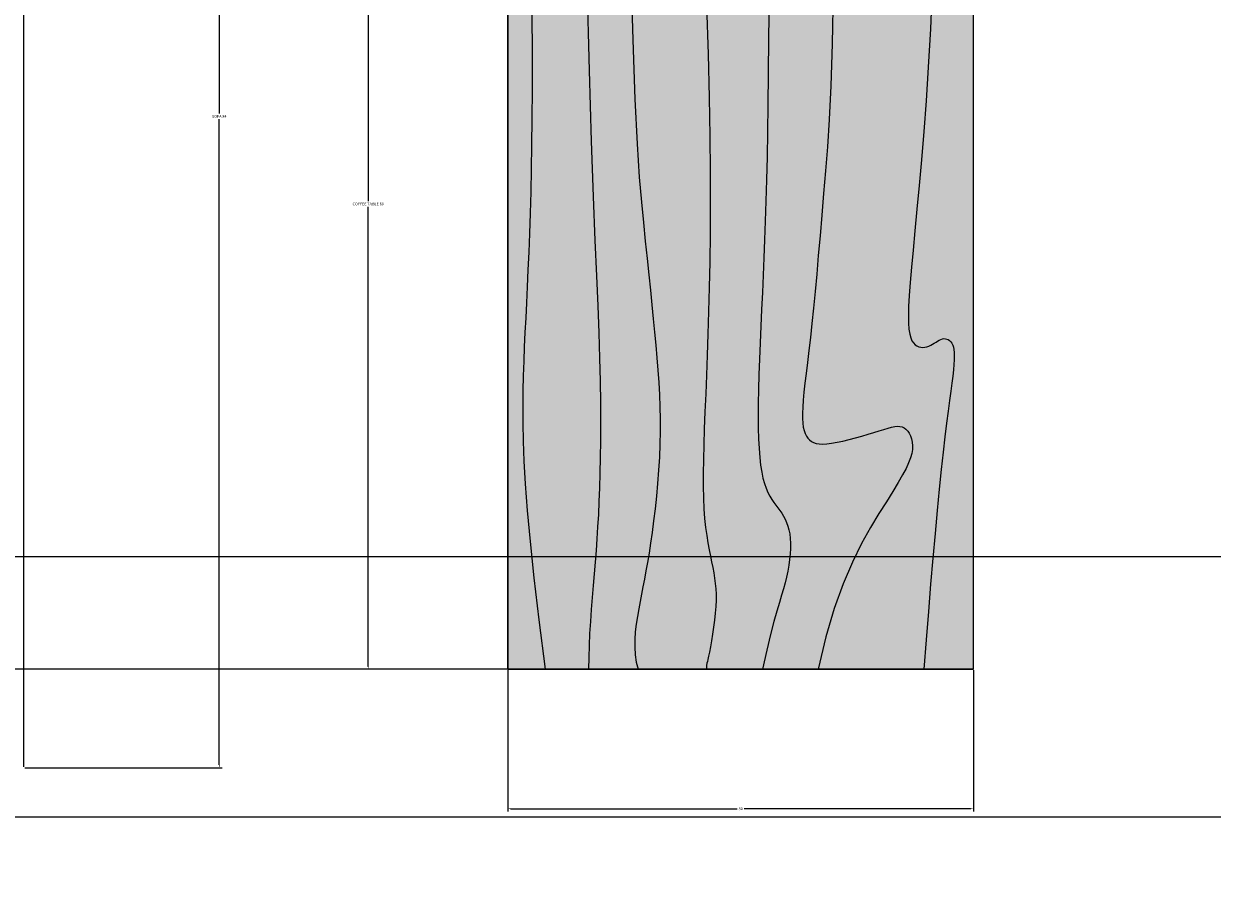
# Model space of a CAD drawing. Units: inches. Extents: x 1201 to 1754, y 247 to 775.
# Tile 3 of 10: x 1305 to 1382, y 435 to 491. Entities that reach past the tile are written whole.
import ezdxf

# ---------------------------------------------------------------- set-up
doc = ezdxf.new("R2010")
doc.units = ezdxf.units.IN
for name, color, linetype, lineweight in [('A-ANNO-DIMS', 2, 'Continuous', 18), ('A-FURN', 8, 'Continuous', 18), ('A-FURN-PATT', 9, 'Continuous', 13)]:
    doc.layers.add(name, color=color, linetype=linetype, lineweight=lineweight)
doc.styles.get("Standard").update_dxf_attribs({"font": 'arial.ttf'})
doc.dimstyles.get("Standard").update_dxf_attribs({"dimtxt": 0.18, "dimasz": 0.18, "dimexe": 0.18, "dimexo": 0.0625, "dimgap": 0.09, "dimtad": 0, "dimtih": 1, "dimtoh": 1, "dimdec": 4, "dimzin": 0, "dimdsep": 46, "dimtxsty": 'Standard', "dimcen": 0.09, "dimadec": 0, "dimazin": 0, "dimtfac": 1, "dimtdec": 4, "dimtofl": 0, "dimtmove": 0, "dimatfit": 3, "dimfxl": 1, "dimtolj": 1, "dimtzin": 0, "dimarcsym": 0})

# ---------------------------------------------------------------- blocks, each defined once
blk = doc.blocks.new('Table - Rectangular Woodgrain 60 x 30 in.')
for p, q in [((0, 0), (0, -30)), ((60, 0), (0, 0)), ((60, -30), (60, 0)), ((0, -30), (60, -30))]:
    blk.add_line(p, q)
for points in [[(0, -2.4), (4.8155, -2.418), (9.0302, -2.4688), (12.709, -2.5477), (15.9167, -2.65), (18.7181, -2.7711), (21.1781, -2.9063), (23.3616, -3.0508), (25.3333, -3.2), (27.1477, -3.3495), (28.8172, -3.4958), (30.3437, -3.636), (31.7291, -3.7667), (32.9756, -3.8849), (34.0849, -3.9875), (35.059, -4.0714), (35.9, -4.1334), (36.6114, -4.1711), (37.2041, -4.1854), (37.6906, -4.1779), (38.0833, -4.15), (38.3948, -4.1034), (38.6375, -4.0396), (38.8239, -3.9602), (38.9666, -3.8667), (39.0764, -3.7608), (39.1573, -3.6448), (39.2116, -3.521), (39.2416, -3.3917), (39.2498, -3.2593), (39.2385, -3.1261), (39.21, -2.9944), (39.1666, -2.8667), (39.111, -2.7447), (39.0468, -2.6281), (38.978, -2.5163), (38.9083, -2.4083), (38.8418, -2.3035), (38.7823, -2.201), (38.7337, -2.1001), (38.7, -2), (38.6844, -1.9003), (38.6875, -1.8021), (38.7094, -1.707), (38.75, -1.6167), (38.8094, -1.5326), (38.8875, -1.4563), (38.9844, -1.3893), (39.1, -1.3333), (39.2351, -1.2896), (39.3937, -1.2583), (39.5804, -1.2396), (39.8, -1.2333), (40.057, -1.2396), (40.3562, -1.2583), (40.7023, -1.2896), (41.1, -1.3333), (41.5547, -1.3895), (42.0755, -1.4573), (42.6721, -1.5361), (43.3542, -1.625), (44.1316, -1.7233), (45.014, -1.8302), (46.0114, -1.9449), (47.1333, -2.0667), (48.3862, -2.1947), (49.7625, -2.3281), (51.2513, -2.4663), (52.8416, -2.6083), (54.5226, -2.7535), (56.2833, -2.9011), (58.1127, -3.0501), (60, -3.2)], [(0, -9.2), (6.5759, -9.0858), (11.9385, -9.0365), (16.2527, -9.0418), (19.6833, -9.0917), (22.3952, -9.1759), (24.5531, -9.2844), (26.322, -9.4069), (27.8666, -9.5333), (29.3241, -9.6553), (30.7203, -9.7719), (32.0532, -9.8837), (33.3208, -9.9917), (34.5213, -10.0965), (35.6526, -10.199), (36.7128, -10.2999), (37.7, -10.4), (38.6129, -10.4996), (39.4531, -10.5969), (40.223, -10.6895), (40.925, -10.775), (41.5613, -10.8512), (42.1344, -10.9156), (42.6465, -10.966), (43.1, -11), (43.4976, -11.0158), (43.8437, -11.0136), (44.143, -10.9942), (44.4, -10.9583), (44.6195, -10.9069), (44.8062, -10.8406), (44.9648, -10.7603), (45.1, -10.6667), (45.2155, -10.5598), (45.3114, -10.4365), (45.3871, -10.2929), (45.4416, -10.125), (45.4743, -9.929), (45.4844, -9.7011), (45.4709, -9.4371), (45.4333, -9.1333), (45.3716, -8.7883), (45.2896, -8.4104), (45.1919, -8.0107), (45.0833, -7.6), (44.9685, -7.1893), (44.8521, -6.7896), (44.7388, -6.4117), (44.6333, -6.0667), (44.54, -5.7628), (44.4614, -5.4979), (44.4001, -5.2675), (44.3583, -5.0667), (44.3384, -4.8909), (44.3427, -4.7354), (44.3736, -4.5956), (44.4333, -4.4667), (44.5236, -4.3453), (44.6427, -4.2333), (44.7884, -4.1339), (44.9583, -4.05), (45.1501, -3.9849), (45.3614, -3.9417), (45.59, -3.9234), (45.8333, -3.9333), (46.0915, -3.9749), (46.3734, -4.0531), (46.6906, -4.1736), (47.0542, -4.3417), (47.4756, -4.5629), (47.9661, -4.8427), (48.5372, -5.1866), (49.2, -5.6), (49.9676, -6.0844), (50.8594, -6.625), (51.8965, -7.2031), (53.1, -7.8), (54.491, -8.3969), (56.0906, -8.975), (57.9199, -9.5156), (60, -10)], [(0, -12.8), (5.1847, -12.9322), (9.6213, -13.0323), (13.3963, -13.1059), (16.5958, -13.1583), (19.3063, -13.1952), (21.614, -13.2219), (23.6054, -13.2439), (25.3666, -13.2667), (26.9728, -13.2947), (28.4531, -13.3281), (29.8256, -13.3663), (31.1083, -13.4083), (32.3191, -13.4535), (33.476, -13.501), (34.597, -13.5501), (35.7, -13.6), (36.7984, -13.6497), (37.8875, -13.6979), (38.9578, -13.743), (40, -13.7833), (41.0047, -13.8174), (41.9625, -13.8438), (42.864, -13.8607), (43.7, -13.8667), (44.4631, -13.8604), (45.1552, -13.8417), (45.7801, -13.8104), (46.3416, -13.7667), (46.8439, -13.7104), (47.2906, -13.6417), (47.6858, -13.5604), (48.0333, -13.4667), (48.3375, -13.3608), (48.6042, -13.2448), (48.8396, -13.121), (49.05, -12.9917), (49.2417, -12.8593), (49.4208, -12.7261), (49.5937, -12.5944), (49.7667, -12.4667), (49.9452, -12.3451), (50.1323, -12.2313), (50.3303, -12.1268), (50.5416, -12.0333), (50.7686, -11.9524), (51.0135, -11.8854), (51.2788, -11.8341), (51.5666, -11.8), (51.8785, -11.7843), (52.2116, -11.7865), (52.562, -11.8059), (52.926, -11.8417), (53.2998, -11.8931), (53.6795, -11.9594), (54.0614, -12.0397), (54.4416, -12.1333), (54.8223, -12.2401), (55.2293, -12.3625), (55.6942, -12.5037), (56.2489, -12.6667), (56.9251, -12.8547), (57.7545, -13.0708), (58.7689, -13.3182), (60, -13.6)], [(0, -18), (5.124, -17.7273), (9.6609, -17.5057), (13.6705, -17.3303), (17.2125, -17.1958), (20.3467, -17.0973), (23.1328, -17.0297), (25.6307, -16.9878), (27.9, -16.9667), (29.9928, -16.9617), (31.9302, -16.9703), (33.7254, -16.9907), (35.3917, -17.0208), (36.9423, -17.0588), (38.3906, -17.1026), (39.7499, -17.1503), (41.0333, -17.2), (42.2519, -17.2496), (43.4073, -17.2969), (44.4986, -17.3395), (45.525, -17.375), (46.4858, -17.4012), (47.3802, -17.4156), (48.2074, -17.416), (48.9667, -17.4), (49.6583, -17.3662), (50.2872, -17.3167), (50.8595, -17.2547), (51.3812, -17.1833), (51.8584, -17.1057), (52.2971, -17.025), (52.7034, -16.9443), (53.0833, -16.8667), (53.443, -16.7951), (53.789, -16.7313), (54.128, -16.6768), (54.4666, -16.6334), (54.8115, -16.6024), (55.1693, -16.5854), (55.5465, -16.5841), (55.95, -16.6), (56.3828, -16.6337), (56.8346, -16.6823), (57.2915, -16.7418), (57.7396, -16.8084), (58.165, -16.878), (58.5539, -16.9469), (58.8924, -17.0111), (59.1666, -17.0667), (59.3679, -17.1107), (59.5078, -17.1438), (59.6032, -17.1675), (59.6708, -17.1833), (59.7275, -17.193), (59.7901, -17.1979), (59.8753, -17.1998), (60, -17.2)], [(0, -22.4), (8.0098, -22.2501), (14.4094, -22.1011), (19.4168, -21.9535), (23.25, -21.8083), (26.1269, -21.6663), (28.2656, -21.5281), (29.884, -21.3947), (31.2, -21.2667), (32.3967, -21.1448), (33.5172, -21.0292), (34.5697, -20.9198), (35.5625, -20.8167), (36.5037, -20.7198), (37.4015, -20.6292), (38.2642, -20.5448), (39.1, -20.4667), (39.9164, -20.3951), (40.7187, -20.3313), (41.5117, -20.2768), (42.3, -20.2333), (43.0883, -20.2024), (43.8812, -20.1854), (44.6836, -20.1841), (45.5, -20.2), (46.3328, -20.234), (47.1747, -20.2844), (48.0163, -20.3488), (48.8479, -20.425), (49.66, -20.5106), (50.4429, -20.6031), (51.1872, -20.7004), (51.8833, -20.8), (52.5246, -20.8999), (53.1166, -20.9995), (53.6681, -21.0983), (54.1875, -21.1958), (54.6834, -21.2919), (55.1646, -21.3859), (55.6394, -21.4777), (56.1167, -21.5667), (56.6028, -21.6515), (57.0961, -21.7266), (57.5929, -21.7852), (58.0896, -21.8208), (58.5823, -21.8268), (59.0674, -21.7964), (59.5412, -21.723), (60, -21.6)], [(0, -25.2), (8.6355, -25.0504), (15.7026, -24.9031), (21.4049, -24.7606), (25.9458, -24.625), (29.529, -24.4988), (32.3578, -24.3844), (34.6359, -24.284), (36.5667, -24.2), (38.3213, -24.1341), (39.9417, -24.0854), (41.437, -24.0523), (42.8167, -24.0333), (44.0901, -24.0268), (45.2667, -24.0313), (46.3557, -24.0451), (47.3667, -24.0667), (48.309, -24.0947), (49.1928, -24.1287), (50.0284, -24.168), (50.826, -24.2125), (51.5959, -24.2617), (52.3483, -24.3151), (53.0935, -24.3725), (53.8417, -24.4334), (54.6009, -24.497), (55.3699, -24.561), (56.1454, -24.6226), (56.9239, -24.6792), (57.7021, -24.7279), (58.4764, -24.7662), (59.2435, -24.7911), (60, -24.8)], [(0, -28.8), (5.6867, -28.6681), (10.45, -28.5698), (14.407, -28.5012), (17.675, -28.4584), (20.3711, -28.4374), (22.6125, -28.4344), (24.5164, -28.4455), (26.2, -28.4667), (27.762, -28.4947), (29.2276, -28.5281), (30.6033, -28.5663), (31.8958, -28.6084), (33.1118, -28.6535), (34.2578, -28.7011), (35.3405, -28.7501), (36.3666, -28.8), (37.3443, -28.8497), (38.288, -28.8974), (39.2137, -28.9412), (40.1375, -28.9792), (41.0753, -29.0093), (42.0432, -29.0297), (43.0572, -29.0384), (44.1333, -29.0333), (45.2936, -29.0114), (46.5843, -28.9641), (48.0579, -28.8816), (49.7666, -28.7542), (51.7629, -28.5721), (54.0989, -28.3255), (56.8272, -28.0048), (60, -27.6)]]:
    blk.add_lwpolyline(points)
blk = doc.blocks.new('*D35')
at = {"layer": 'A-ANNO-DIMS', "color": 0, "lineweight": -2, "transparency": 16777216}
for p, q in [((1336.149, 509.584), (1327.031, 509.584)), ((1327.211, 509.404), (1327.211, 479.767)), ((1327.211, 449.764), (1327.211, 479.401)), ((1336.149, 449.584), (1327.031, 449.584))]:
    blk.add_line(p, q, dxfattribs=at)
at = {"layer": 'A-ANNO-DIMS', "color": 0, "transparency": 16777216}
for points in [[(1327.181, 509.404), (1327.241, 509.404), (1327.211, 509.584)], [(1327.181, 449.764), (1327.241, 449.764), (1327.211, 449.584)]]:
    blk.add_solid(points, dxfattribs=at)
at = {"layer": 'Defpoints', "color": 0, "transparency": 16777216}
for p in [(1336.211, 509.584), (1327.211, 449.584), (1336.211, 449.584)]:
    blk.add_point(p, dxfattribs=at)
at = {"layer": 'A-ANNO-DIMS', "color": 0, "transparency": 16777216, "insert": (1327.211, 479.584), "char_height": 0.18, "attachment_point": 5}
blk.add_mtext('\\A1;COFFEE TABLE 60', dxfattribs=at)
blk = doc.blocks.new('*D36')
at = {"layer": 'A-ANNO-DIMS', "color": 0, "lineweight": -2, "transparency": 16777216}
for p, q in [((1336.211, 449.521), (1336.211, 440.404)), ((1366.211, 449.521), (1366.211, 440.404)), ((1336.391, 440.584), (1350.993, 440.584)), ((1366.031, 440.584), (1351.43, 440.584))]:
    blk.add_line(p, q, dxfattribs=at)
at = {"layer": 'A-ANNO-DIMS', "color": 0, "transparency": 16777216}
for points in [[(1336.391, 440.614), (1336.391, 440.554), (1336.211, 440.584)], [(1366.031, 440.614), (1366.031, 440.554), (1366.211, 440.584)]]:
    blk.add_solid(points, dxfattribs=at)
at = {"layer": 'Defpoints', "color": 0, "transparency": 16777216}
for p in [(1336.211, 449.584), (1366.211, 449.584), (1366.211, 440.584)]:
    blk.add_point(p, dxfattribs=at)
at = {"layer": 'A-ANNO-DIMS', "color": 0, "transparency": 16777216, "insert": (1351.211, 440.584), "char_height": 0.18, "attachment_point": 5}
blk.add_mtext('\\A1;30', dxfattribs=at)
blk = doc.blocks.new('*D37')
at = {"layer": 'A-ANNO-DIMS', "color": 0, "lineweight": -2, "transparency": 16777216}
for p, q in [((1305.079, 527.227), (1317.797, 527.227)), ((1317.617, 527.047), (1317.617, 485.41)), ((1317.617, 443.407), (1317.617, 485.044)), ((1305.079, 443.227), (1317.797, 443.227))]:
    blk.add_line(p, q, dxfattribs=at)
at = {"layer": 'A-ANNO-DIMS', "color": 0, "transparency": 16777216}
for points in [[(1317.587, 527.047), (1317.647, 527.047), (1317.617, 527.227)], [(1317.587, 443.407), (1317.647, 443.407), (1317.617, 443.227)]]:
    blk.add_solid(points, dxfattribs=at)
at = {"layer": 'Defpoints', "color": 0, "transparency": 16777216}
for p in [(1305.017, 527.227), (1317.617, 527.227), (1305.017, 443.227)]:
    blk.add_point(p, dxfattribs=at)
at = {"layer": 'A-ANNO-DIMS', "color": 0, "transparency": 16777216, "insert": (1317.617, 485.227), "char_height": 0.18, "attachment_point": 5}
blk.add_mtext('\\A1;SOFA 84', dxfattribs=at)
blk = doc.blocks.new('*D59')
at = {"layer": 'A-ANNO-DIMS', "color": 0, "lineweight": -2, "transparency": 16777216}
for p, q in [((1255.521, 418.004), (1255.521, 775.136)), ((1405.521, 418.004), (1405.521, 775.136)), ((1255.701, 774.956), (1330.241, 774.956)), ((1405.341, 774.956), (1330.801, 774.956))]:
    blk.add_line(p, q, dxfattribs=at)
at = {"layer": 'A-ANNO-DIMS', "color": 0, "transparency": 16777216}
for points in [[(1255.701, 774.986), (1255.701, 774.926), (1255.521, 774.956)], [(1405.341, 774.986), (1405.341, 774.926), (1405.521, 774.956)]]:
    blk.add_solid(points, dxfattribs=at)
at = {"layer": 'Defpoints', "color": 0, "transparency": 16777216}
for p in [(1405.521, 774.956), (1255.521, 417.941), (1405.521, 417.941)]:
    blk.add_point(p, dxfattribs=at)
at = {"layer": 'A-ANNO-DIMS', "color": 0, "transparency": 16777216, "insert": (1330.521, 774.956), "char_height": 0.18, "attachment_point": 5}
blk.add_mtext('\\A1;150', dxfattribs=at)
blk = doc.blocks.new('*D94')
at = {"layer": 'A-ANNO-DIMS', "color": 0, "lineweight": -2, "transparency": 16777216}
for p, q in [((1305.017, 443.289), (1305.017, 775.136)), ((1336.211, 449.646), (1336.211, 775.136)), ((1305.197, 774.956), (1320.15, 774.956)), ((1336.031, 774.956), (1321.078, 774.956))]:
    blk.add_line(p, q, dxfattribs=at)
at = {"layer": 'A-ANNO-DIMS', "color": 0, "transparency": 16777216}
for points in [[(1305.197, 774.986), (1305.197, 774.926), (1305.017, 774.956)], [(1336.031, 774.986), (1336.031, 774.926), (1336.211, 774.956)]]:
    blk.add_solid(points, dxfattribs=at)
at = {"layer": 'Defpoints', "color": 0, "transparency": 16777216}
for p in [(1336.211, 774.956), (1336.211, 449.584), (1305.017, 443.227)]:
    blk.add_point(p, dxfattribs=at)
at = {"layer": 'A-ANNO-DIMS', "color": 0, "transparency": 16777216, "insert": (1320.614, 774.956), "char_height": 0.18, "attachment_point": 5}
blk.add_mtext('\\A1;31.195', dxfattribs=at)
blk = doc.blocks.new('*D95')
at = {"layer": 'A-ANNO-DIMS', "color": 0, "lineweight": -2, "transparency": 16777216}
for p, q in [((1366.149, 449.584), (1222.326, 449.584)), ((1222.506, 449.404), (1222.506, 433.945)), ((1222.506, 418.121), (1222.506, 433.581)), ((1405.458, 417.941), (1222.326, 417.941))]:
    blk.add_line(p, q, dxfattribs=at)
at = {"layer": 'A-ANNO-DIMS', "color": 0, "transparency": 16777216}
for points in [[(1222.476, 449.404), (1222.536, 449.404), (1222.506, 449.584)], [(1222.476, 418.121), (1222.536, 418.121), (1222.506, 417.941)]]:
    blk.add_solid(points, dxfattribs=at)
at = {"layer": 'Defpoints', "color": 0, "transparency": 16777216}
for p in [(1366.211, 449.584), (1222.506, 417.941), (1405.521, 417.941)]:
    blk.add_point(p, dxfattribs=at)
at = {"layer": 'A-ANNO-DIMS', "color": 0, "transparency": 16777216, "insert": (1222.506, 433.763), "char_height": 0.18, "attachment_point": 5}
blk.add_mtext('\\A1;31.64', dxfattribs=at)
blk = doc.blocks.new('*D96')
at = {"layer": 'A-ANNO-DIMS', "color": 0, "lineweight": -2, "transparency": 16777216}
for p, q in [((1714.984, 456.827), (1222.326, 456.827)), ((1222.506, 456.647), (1222.506, 448.613)), ((1222.506, 440.214), (1222.506, 448.249)), ((1717.458, 440.034), (1222.326, 440.034))]:
    blk.add_line(p, q, dxfattribs=at)
at = {"layer": 'A-ANNO-DIMS', "color": 0, "transparency": 16777216}
for points in [[(1222.476, 456.647), (1222.536, 456.647), (1222.506, 456.827)], [(1222.476, 440.214), (1222.536, 440.214), (1222.506, 440.034)]]:
    blk.add_solid(points, dxfattribs=at)
at = {"layer": 'Defpoints', "color": 0, "transparency": 16777216}
for p in [(1222.506, 456.827), (1715.047, 456.827), (1717.521, 440.034)]:
    blk.add_point(p, dxfattribs=at)
at = {"layer": 'A-ANNO-DIMS', "color": 0, "transparency": 16777216, "insert": (1222.506, 448.431), "char_height": 0.18, "attachment_point": 5}
blk.add_mtext('\\A1;16.793', dxfattribs=at)
blk = doc.blocks.new('*D100')
at = {"layer": 'A-ANNO-DIMS', "color": 0, "lineweight": -2, "transparency": 16777216}
for p, q in [((1204.298, 485.227), (1276.837, 485.227)), ((1398.123, 485.227), (1398.303, 485.227)), ((1398.213, 485.137), (1398.213, 485.317))]:
    blk.add_line(p, q, dxfattribs=at)
at = {"layer": 'A-ANNO-DIMS', "color": 0, "transparency": 16777216}
blk.add_solid([(1276.837, 485.257), (1276.837, 485.197), (1277.017, 485.227)], dxfattribs=at)
at = {"layer": 'Defpoints', "color": 0, "transparency": 16777216}
for p in [(1277.017, 485.227), (1398.213, 485.227)]:
    blk.add_point(p, dxfattribs=at)
at = {"layer": 'A-ANNO-DIMS', "color": 0, "transparency": 16777216, "insert": (1203.82, 485.227), "char_height": 0.18, "attachment_point": 5}
blk.add_mtext('\\A1;R121.2', dxfattribs=at)
blk = doc.blocks.new('*D101')
at = {"layer": 'A-ANNO-DIMS', "color": 0, "lineweight": -2, "transparency": 16777216}
for p, q in [((1202.467, 485.227), (1270.837, 485.227)), ((1385.177, 485.227), (1385.357, 485.227)), ((1385.267, 485.137), (1385.267, 485.317))]:
    blk.add_line(p, q, dxfattribs=at)
at = {"layer": 'A-ANNO-DIMS', "color": 0, "transparency": 16777216}
blk.add_solid([(1270.837, 485.257), (1270.837, 485.197), (1271.017, 485.227)], dxfattribs=at)
at = {"layer": 'Defpoints', "color": 0, "transparency": 16777216}
for p in [(1271.017, 485.227), (1385.267, 485.227)]:
    blk.add_point(p, dxfattribs=at)
at = {"layer": 'A-ANNO-DIMS', "color": 0, "transparency": 16777216, "insert": (1201.916, 485.227), "char_height": 0.18, "attachment_point": 5}
blk.add_mtext('\\A1;R114.25', dxfattribs=at)

msp = doc.modelspace()

# ---------------------------------------------------------------- hatches: boundary and pattern name
at = {"layer": 'A-FURN-PATT'}
h = msp.add_hatch(color=256, dxfattribs=at)
h.dxf.hatch_style = 1
h.paths.add_polyline_path([(1363.7933, 504.7684), (1363.8113, 509.5839), (1357.0113, 509.5839), (1357.1255, 503.008), (1357.1748, 497.6454), (1357.1695, 493.3312), (1357.1196, 489.9006), (1357.0354, 487.1887), (1356.9269, 485.0308), (1356.8044, 483.2619), (1356.678, 481.7173), (1356.556, 480.2598), (1356.4394, 478.8636), (1356.3276, 477.5307), (1356.2196, 476.2631), (1356.1148, 475.0626), (1356.0123, 473.9313), (1355.9114, 472.8711), (1355.8113, 471.8839), (1355.7117, 470.971), (1355.6144, 470.1308), (1355.5218, 469.3609), (1355.4363, 468.6589), (1355.3601, 468.0226), (1355.2957, 467.4495), (1355.2453, 466.9374), (1355.2113, 466.4839), (1355.1955, 466.0863), (1355.1977, 465.7402), (1355.2171, 465.4409), (1355.253, 465.1839), (1355.3044, 464.9644), (1355.3707, 464.7777), (1355.451, 464.6191), (1355.5446, 464.4839), (1355.6515, 464.3684), (1355.7748, 464.2725), (1355.9184, 464.1968), (1356.0863, 464.1423), (1356.2823, 464.1096), (1356.5102, 464.0995), (1356.7742, 464.113), (1357.078, 464.1506), (1357.423, 464.2123), (1357.8009, 464.2943), (1358.2006, 464.392), (1358.6113, 464.5006), (1359.022, 464.6154), (1359.4217, 464.7318), (1359.7996, 464.8451), (1360.1446, 464.9506), (1360.4485, 465.0439), (1360.7134, 465.1225), (1360.9438, 465.1838), (1361.1446, 465.2256), (1361.3204, 465.2455), (1361.4759, 465.2412), (1361.6157, 465.2103), (1361.7446, 465.1506), (1361.866, 465.0603), (1361.978, 464.9412), (1362.0774, 464.7955), (1362.1613, 464.6256), (1362.2264, 464.4338), (1362.2696, 464.2225), (1362.2879, 463.9939), (1362.278, 463.7506), (1362.2364, 463.4924), (1362.1582, 463.2105), (1362.0377, 462.8933), (1361.8696, 462.5297), (1361.6484, 462.1083), (1361.3686, 461.6178), (1361.0247, 461.0467), (1360.6113, 460.3839), (1360.1269, 459.6163), (1359.5863, 458.7245), (1359.0082, 457.6874), (1358.4113, 456.4839), (1357.8144, 455.0929), (1357.2363, 453.4933), (1356.6957, 451.664), (1356.2113, 449.5839), (1363.0113, 449.5839), (1363.1612, 451.4712), (1363.3102, 453.3006), (1363.4578, 455.0613), (1363.603, 456.7423), (1363.745, 458.3326), (1363.8832, 459.8214), (1364.0166, 461.1977), (1364.1446, 462.4506), (1364.2664, 463.5725), (1364.3811, 464.5699), (1364.488, 465.4523), (1364.5863, 466.2297), (1364.6752, 466.9118), (1364.754, 467.5084), (1364.8218, 468.0292), (1364.878, 468.4839), (1364.9217, 468.8816), (1364.953, 469.2277), (1364.9717, 469.5269), (1364.978, 469.7839), (1364.9717, 470.0035), (1364.953, 470.1902), (1364.9217, 470.3488), (1364.878, 470.4839), (1364.822, 470.5995), (1364.755, 470.6964), (1364.6787, 470.7745), (1364.5946, 470.8339), (1364.5043, 470.8745), (1364.4092, 470.8964), (1364.311, 470.8995), (1364.2113, 470.8839), (1364.1112, 470.8502), (1364.0103, 470.8016), (1363.9078, 470.7421), (1363.803, 470.6756), (1363.6186, 470.5566), (1363.3995, 470.436), (1363.149, 470.3508), (1362.881, 470.3281), (1362.6903, 470.3723), (1362.5665, 470.4266), (1362.4505, 470.5075), (1362.3446, 470.6173), (1362.2511, 470.76), (1362.1717, 470.9464), (1362.1079, 471.1891), (1362.0613, 471.5006), (1362.0334, 471.8933), (1362.0259, 472.3798), (1362.0402, 472.9725), (1362.0779, 473.6839), (1362.1399, 474.5249), (1362.2238, 475.499), (1362.3264, 476.6083), (1362.4446, 477.8548), (1362.5753, 479.2402), (1362.7155, 480.7667), (1362.8618, 482.4362), (1363.0113, 484.2506), (1363.1605, 486.2223), (1363.305, 488.4058), (1363.4402, 490.8658), (1363.5613, 493.6672), (1363.6636, 496.8749), (1363.7425, 500.5537)])
h.paths.add_polyline_path([(1342.1259, 469.6422), (1342.0772, 471.2626), (1342.0113, 473.0172), (1341.9273, 474.948), (1341.8269, 477.2261), (1341.7125, 480.0549), (1341.5863, 483.6381), (1341.4507, 488.179), (1341.3082, 493.8813), (1341.1609, 500.9484), (1341.0113, 509.5839), (1337.4113, 509.5839), (1337.5432, 503.8972), (1337.6415, 499.1339), (1337.7101, 495.1769), (1337.7529, 491.9089), (1337.7739, 489.2128), (1337.7769, 486.9714), (1337.7658, 485.0675), (1337.7446, 483.3839), (1337.7166, 481.8219), (1337.6832, 480.3563), (1337.645, 478.9806), (1337.6029, 477.6881), (1337.5578, 476.4721), (1337.5102, 475.3261), (1337.4612, 474.2434), (1337.4113, 473.2173), (1337.3616, 472.2396), (1337.3139, 471.2959), (1337.2701, 470.3702), (1337.2321, 469.4464), (1337.202, 468.5086), (1337.1816, 467.5407), (1337.1729, 466.5267), (1337.178, 465.4506), (1337.1999, 464.2903), (1337.2472, 462.9996), (1337.3297, 461.526), (1337.4571, 459.8173), (1337.6392, 457.821), (1337.8858, 455.485), (1338.2065, 452.7567), (1338.6113, 449.5839), (1341.4113, 449.5839), (1341.4202, 450.3404), (1341.4451, 451.1075), (1341.4834, 451.8818), (1341.5321, 452.66), (1341.5887, 453.4385), (1341.6503, 454.214), (1341.7143, 454.983), (1341.7779, 455.7422), (1341.8388, 456.4904), (1341.8962, 457.2356), (1341.9496, 457.988), (1341.9988, 458.7579), (1342.0433, 459.5555), (1342.0826, 460.3911), (1342.1166, 461.2749), (1342.1446, 462.2172), (1342.1662, 463.2282), (1342.18, 464.3172), (1342.1845, 465.4938), (1342.178, 466.7672), (1342.159, 468.1469)])
h.paths.add_polyline_path([(1345.8625, 461.5676), (1345.9269, 462.4092), (1345.9773, 463.2511), (1346.0113, 464.0839), (1346.0272, 464.9003), (1346.0259, 465.7027), (1346.0089, 466.4956), (1345.978, 467.2839), (1345.9345, 468.0722), (1345.88, 468.8652), (1345.8162, 469.6675), (1345.7446, 470.4839), (1345.6665, 471.3197), (1345.5821, 472.1824), (1345.4915, 473.0802), (1345.3946, 474.0214), (1345.2915, 475.0142), (1345.1821, 476.0667), (1345.0665, 477.1872), (1344.9446, 478.3839), (1344.8166, 479.6999), (1344.6832, 481.3183), (1344.545, 483.457), (1344.403, 486.3339), (1344.2578, 490.1671), (1344.1102, 495.1745), (1343.9612, 501.5741), (1343.8113, 509.5839), (1341.0113, 509.5839), (1341.1609, 500.9484), (1341.3082, 493.8813), (1341.4507, 488.179), (1341.5863, 483.6381), (1341.7125, 480.0549), (1341.8269, 477.2261), (1341.9273, 474.948), (1342.0113, 473.0172), (1342.0772, 471.2626), (1342.1259, 469.6422), (1342.159, 468.1469), (1342.178, 466.7672), (1342.1845, 465.4938), (1342.18, 464.3172), (1342.1662, 463.2282), (1342.1446, 462.2172), (1342.1166, 461.2749), (1342.0826, 460.3911), (1342.0433, 459.5555), (1341.9988, 458.7579), (1341.9496, 457.988), (1341.8962, 457.2356), (1341.8388, 456.4904), (1341.7779, 455.7422), (1341.7143, 454.983), (1341.6503, 454.214), (1341.5887, 453.4385), (1341.5321, 452.66), (1341.4834, 451.8818), (1341.4451, 451.1075), (1341.4202, 450.3404), (1341.4113, 449.5839), (1344.6113, 449.5839), (1344.4883, 450.0427), (1344.4149, 450.5165), (1344.3845, 451.0016), (1344.3905, 451.4943), (1344.4261, 451.991), (1344.4847, 452.4878), (1344.5598, 452.9811), (1344.6446, 453.4672), (1344.7336, 453.9445), (1344.8254, 454.4193), (1344.9194, 454.9005), (1345.0155, 455.3964), (1345.113, 455.9158), (1345.2118, 456.4673), (1345.3114, 457.0593), (1345.4113, 457.7006), (1345.5109, 458.3967), (1345.6082, 459.141), (1345.7007, 459.9239), (1345.7863, 460.736)])
h.paths.add_polyline_path([(1349.1056, 457.7255), (1349.028, 458.2027), (1348.9566, 458.7244), (1348.8946, 459.2967), (1348.8451, 459.9256), (1348.8113, 460.6172), (1348.7953, 461.3765), (1348.7957, 462.2037), (1348.8101, 463.0981), (1348.8363, 464.0589), (1348.8718, 465.0853), (1348.9144, 466.1766), (1348.9617, 467.332), (1349.0113, 468.5506), (1349.061, 469.834), (1349.1087, 471.1933), (1349.1525, 472.6416), (1349.1905, 474.1922), (1349.2206, 475.8585), (1349.241, 477.6537), (1349.2496, 479.5911), (1349.2446, 481.6839), (1349.2235, 483.9532), (1349.1816, 486.4511), (1349.114, 489.2372), (1349.0155, 492.3714), (1348.881, 495.9134), (1348.7056, 499.923), (1348.484, 504.4599), (1348.2113, 509.5839), (1343.8113, 509.5839), (1343.9612, 501.5741), (1344.1102, 495.1745), (1344.2578, 490.1671), (1344.403, 486.3339), (1344.545, 483.457), (1344.6832, 481.3183), (1344.8166, 479.6999), (1344.9446, 478.3839), (1345.0665, 477.1872), (1345.1821, 476.0667), (1345.2915, 475.0142), (1345.3946, 474.0214), (1345.4915, 473.0802), (1345.5821, 472.1824), (1345.6665, 471.3197), (1345.7446, 470.4839), (1345.8162, 469.6675), (1345.88, 468.8652), (1345.9345, 468.0722), (1345.978, 467.2839), (1346.0089, 466.4956), (1346.0259, 465.7027), (1346.0272, 464.9003), (1346.0113, 464.0839), (1345.9773, 463.2511), (1345.9269, 462.4092), (1345.8625, 461.5676), (1345.7863, 460.736), (1345.7007, 459.9239), (1345.6082, 459.141), (1345.5109, 458.3967), (1345.4113, 457.7006), (1345.3114, 457.0593), (1345.2118, 456.4673), (1345.113, 455.9158), (1345.0155, 455.3964), (1344.9194, 454.9005), (1344.8254, 454.4193), (1344.7336, 453.9445), (1344.6446, 453.4672), (1344.5598, 452.9811), (1344.4847, 452.4878), (1344.4261, 451.991), (1344.3905, 451.4943), (1344.3845, 451.0016), (1344.4149, 450.5165), (1344.4883, 450.0427), (1344.6113, 449.5839), (1349.0113, 449.5839), (1349.0117, 449.8177), (1349.0302, 449.9259), (1349.0675, 450.0761), (1349.1006, 450.216), (1349.1446, 450.4173), (1349.2002, 450.6915), (1349.2644, 451.03), (1349.3333, 451.4189), (1349.4029, 451.8443), (1349.4695, 452.2924), (1349.529, 452.7493), (1349.5776, 453.2011), (1349.6113, 453.6339), (1349.6272, 454.0374), (1349.6259, 454.4146), (1349.6089, 454.7724), (1349.5779, 455.1173), (1349.5345, 455.4559), (1349.48, 455.7949), (1349.4162, 456.1409), (1349.3446, 456.5006), (1349.267, 456.8805), (1349.1863, 457.2868)])
h.paths.add_polyline_path([(1354.4248, 457.3723), (1354.427, 457.7054), (1354.4113, 458.0173), (1354.3772, 458.3051), (1354.3259, 458.5704), (1354.2589, 458.8153), (1354.178, 459.0423), (1354.0845, 459.2536), (1353.98, 459.4516), (1353.8662, 459.6387), (1353.7446, 459.8172), (1353.6169, 459.9902), (1353.4852, 460.1631), (1353.352, 460.3422), (1353.2196, 460.5339), (1353.0903, 460.7443), (1352.9665, 460.9797), (1352.8505, 461.2464), (1352.7446, 461.5506), (1352.6509, 461.8981), (1352.5696, 462.2933), (1352.5009, 462.74), (1352.4446, 463.2423), (1352.4009, 463.8038), (1352.3696, 464.4287), (1352.3509, 465.1208), (1352.3446, 465.8839), (1352.3506, 466.7199), (1352.3675, 467.6214), (1352.3939, 468.5792), (1352.428, 469.5839), (1352.4683, 470.6261), (1352.5134, 471.6964), (1352.5616, 472.7855), (1352.6113, 473.8839), (1352.6612, 474.9869), (1352.7103, 476.1079), (1352.7578, 477.2648), (1352.803, 478.4756), (1352.845, 479.7583), (1352.8832, 481.1308), (1352.9166, 482.6111), (1352.9446, 484.2173), (1352.9674, 485.9785), (1352.9894, 487.9699), (1353.0161, 490.2776), (1353.053, 492.9881), (1353.1054, 496.1876), (1353.179, 499.9626), (1353.2791, 504.3992), (1353.4113, 509.5839), (1348.2113, 509.5839), (1348.484, 504.4599), (1348.7056, 499.923), (1348.881, 495.9134), (1349.0155, 492.3714), (1349.114, 489.2372), (1349.1816, 486.4511), (1349.2235, 483.9532), (1349.2446, 481.6839), (1349.2496, 479.5911), (1349.241, 477.6537), (1349.2206, 475.8585), (1349.1905, 474.1922), (1349.1525, 472.6416), (1349.1087, 471.1933), (1349.061, 469.834), (1349.0113, 468.5506), (1348.9617, 467.332), (1348.9144, 466.1766), (1348.8718, 465.0853), (1348.8363, 464.0589), (1348.8101, 463.0981), (1348.7957, 462.2037), (1348.7953, 461.3765), (1348.8113, 460.6172), (1348.8451, 459.9256), (1348.8946, 459.2967), (1348.9566, 458.7244), (1349.028, 458.2027), (1349.1056, 457.7255), (1349.1863, 457.2868), (1349.267, 456.8805), (1349.3446, 456.5006), (1349.4162, 456.1409), (1349.48, 455.7949), (1349.5345, 455.4559), (1349.5779, 455.1173), (1349.6089, 454.7724), (1349.6259, 454.4146), (1349.6272, 454.0374), (1349.6113, 453.6339), (1349.5776, 453.2011), (1349.529, 452.7493), (1349.4695, 452.2924), (1349.4029, 451.8443), (1349.3333, 451.4189), (1349.2644, 451.03), (1349.2002, 450.6915), (1349.1446, 450.4173), (1349.1006, 450.216), (1349.0675, 450.0761), (1349.0438, 449.9807), (1349.028, 449.9131), (1349.0183, 449.8564), (1349.0134, 449.7938), (1349.0115, 449.7086), (1349.0113, 449.5839), (1352.6113, 449.5839), (1352.8931, 450.815), (1353.1405, 451.8294), (1353.3566, 452.6588), (1353.5446, 453.335), (1353.7076, 453.8897), (1353.8488, 454.3546), (1353.9712, 454.7616), (1354.078, 455.1423), (1354.1716, 455.5225), (1354.2519, 455.9044), (1354.3182, 456.2841), (1354.3696, 456.6579), (1354.4054, 457.0219)])
h.paths.add_polyline_path([(1360.1269, 459.6163), (1360.6113, 460.3839), (1361.0247, 461.0467), (1361.3686, 461.6178), (1361.6484, 462.1083), (1361.8696, 462.5297), (1362.0377, 462.8933), (1362.1582, 463.2105), (1362.2364, 463.4924), (1362.278, 463.7506), (1362.2879, 463.9939), (1362.2696, 464.2225), (1362.2264, 464.4338), (1362.1613, 464.6256), (1362.0774, 464.7955), (1361.978, 464.9412), (1361.866, 465.0603), (1361.7446, 465.1506), (1361.6157, 465.2103), (1361.4759, 465.2412), (1361.3204, 465.2455), (1361.1446, 465.2256), (1360.9438, 465.1838), (1360.7134, 465.1225), (1360.4485, 465.0439), (1360.1446, 464.9506), (1359.7996, 464.8451), (1359.4217, 464.7318), (1359.022, 464.6154), (1358.6113, 464.5006), (1358.2006, 464.392), (1357.8009, 464.2943), (1357.423, 464.2123), (1357.078, 464.1506), (1356.7742, 464.113), (1356.5102, 464.0995), (1356.2823, 464.1096), (1356.0863, 464.1423), (1355.9184, 464.1968), (1355.7748, 464.2725), (1355.6515, 464.3684), (1355.5446, 464.4839), (1355.451, 464.6191), (1355.3707, 464.7777), (1355.3044, 464.9644), (1355.253, 465.1839), (1355.2171, 465.4409), (1355.1977, 465.7402), (1355.1955, 466.0863), (1355.2113, 466.4839), (1355.2453, 466.9374), (1355.2957, 467.4495), (1355.3601, 468.0226), (1355.4363, 468.6589), (1355.5218, 469.3609), (1355.6144, 470.1308), (1355.7117, 470.971), (1355.8113, 471.8839), (1355.9114, 472.8711), (1356.0123, 473.9313), (1356.1148, 475.0626), (1356.2196, 476.2631), (1356.3276, 477.5307), (1356.4394, 478.8636), (1356.556, 480.2598), (1356.678, 481.7173), (1356.8044, 483.2619), (1356.9269, 485.0308), (1357.0354, 487.1887), (1357.1196, 489.9006), (1357.1695, 493.3312), (1357.1748, 497.6454), (1357.1255, 503.008), (1357.0113, 509.5839), (1353.4113, 509.5839), (1353.2791, 504.3992), (1353.179, 499.9626), (1353.1054, 496.1876), (1353.053, 492.9881), (1353.0161, 490.2776), (1352.9894, 487.9699), (1352.9674, 485.9785), (1352.9446, 484.2173), (1352.9166, 482.6111), (1352.8832, 481.1308), (1352.845, 479.7583), (1352.803, 478.4756), (1352.7578, 477.2648), (1352.7103, 476.1079), (1352.6612, 474.9869), (1352.6113, 473.8839), (1352.5616, 472.7855), (1352.5134, 471.6964), (1352.4683, 470.6261), (1352.428, 469.5839), (1352.3939, 468.5792), (1352.3675, 467.6214), (1352.3506, 466.7199), (1352.3446, 465.8839), (1352.3509, 465.1208), (1352.3696, 464.4287), (1352.4009, 463.8038), (1352.4446, 463.2423), (1352.5009, 462.74), (1352.5696, 462.2933), (1352.6509, 461.8981), (1352.7446, 461.5506), (1352.8505, 461.2464), (1352.9665, 460.9797), (1353.0903, 460.7443), (1353.2196, 460.5339), (1353.352, 460.3422), (1353.4852, 460.1631), (1353.6169, 459.9902), (1353.7446, 459.8172), (1353.8662, 459.6387), (1353.98, 459.4516), (1354.0845, 459.2536), (1354.178, 459.0423), (1354.2589, 458.8153), (1354.3259, 458.5704), (1354.3772, 458.3051), (1354.4113, 458.0173), (1354.427, 457.7054), (1354.4248, 457.3723), (1354.4054, 457.0219), (1354.3696, 456.6579), (1354.3182, 456.2841), (1354.2519, 455.9044), (1354.1716, 455.5225), (1354.078, 455.1423), (1353.9712, 454.7616), (1353.8488, 454.3546), (1353.7076, 453.8897), (1353.5446, 453.335), (1353.3566, 452.6588), (1353.1405, 451.8294), (1352.8931, 450.815), (1352.6113, 449.5839), (1356.2113, 449.5839), (1356.6957, 451.664), (1357.2363, 453.4933), (1357.8144, 455.0929), (1358.4113, 456.4839), (1359.0082, 457.6874), (1359.5863, 458.7245)])
h.paths.add_polyline_path([(1366.2113, 509.5839), (1363.8113, 509.5839), (1363.7933, 504.7684), (1363.7425, 500.5537), (1363.6636, 496.8749), (1363.5613, 493.6672), (1363.4402, 490.8658), (1363.305, 488.4058), (1363.1605, 486.2223), (1363.0113, 484.2506), (1362.8618, 482.4362), (1362.7155, 480.7667), (1362.5753, 479.2402), (1362.4446, 477.8548), (1362.3264, 476.6083), (1362.2238, 475.499), (1362.1399, 474.5249), (1362.0779, 473.6839), (1362.0402, 472.9725), (1362.0259, 472.3798), (1362.0334, 471.8933), (1362.0613, 471.5006), (1362.1079, 471.1891), (1362.1717, 470.9464), (1362.2511, 470.76), (1362.3446, 470.6173), (1362.4505, 470.5075), (1362.5665, 470.4266), (1362.6903, 470.3723), (1362.8196, 470.3423), (1362.952, 470.3341), (1363.0852, 470.3454), (1363.2169, 470.3739), (1363.3446, 470.4173), (1363.4666, 470.4729), (1363.5832, 470.5371), (1363.695, 470.6059), (1363.8903, 470.7319), (1364.0703, 470.8364), (1364.2622, 470.901), (1364.4591, 470.8948), (1364.6411, 470.813), (1364.7948, 470.6557), (1364.878, 470.4839), (1364.9217, 470.3488), (1364.953, 470.1902), (1364.9717, 470.0035), (1364.978, 469.7839), (1364.9717, 469.5269), (1364.953, 469.2277), (1364.9217, 468.8816), (1364.878, 468.4839), (1364.8218, 468.0292), (1364.754, 467.5084), (1364.6752, 466.9118), (1364.5863, 466.2297), (1364.488, 465.4523), (1364.3811, 464.5699), (1364.2664, 463.5725), (1364.1446, 462.4506), (1364.0166, 461.1977), (1363.8832, 459.8214), (1363.745, 458.3326), (1363.603, 456.7423), (1363.4578, 455.0613), (1363.3102, 453.3006), (1363.1612, 451.4712), (1363.0113, 449.5839), (1366.2113, 449.5839)])
h.paths.add_polyline_path([(1338.2065, 452.7567), (1337.8858, 455.485), (1337.6392, 457.821), (1337.4571, 459.8173), (1337.3297, 461.526), (1337.2472, 462.9996), (1337.1999, 464.2903), (1337.178, 465.4506), (1337.1729, 466.5267), (1337.1816, 467.5407), (1337.202, 468.5086), (1337.2321, 469.4464), (1337.2701, 470.3702), (1337.3139, 471.2959), (1337.3616, 472.2396), (1337.4113, 473.2173), (1337.4612, 474.2434), (1337.5102, 475.3261), (1337.5578, 476.4721), (1337.6029, 477.6881), (1337.645, 478.9806), (1337.6832, 480.3563), (1337.7166, 481.8219), (1337.7446, 483.3839), (1337.7658, 485.0675), (1337.7769, 486.9714), (1337.7739, 489.2128), (1337.7529, 491.9089), (1337.7101, 495.1769), (1337.6415, 499.1339), (1337.5432, 503.8972), (1337.4113, 509.5839), (1336.2113, 509.5839), (1336.2113, 449.5839), (1338.6113, 449.5839)])

# ---------------------------------------------------------------- block references
at = {"layer": 'A-FURN', "rotation": 270}
msp.add_blockref('Table - Rectangular Woodgrain 60 x 30 in.', (1366.2113, 509.5839), dxfattribs=at)

# ---------------------------------------------------------------- dimensions: what is measured, and where the dimension line sits
at = {"layer": 'A-ANNO-DIMS'}
for base, p1, p2, override, picture, middle in [((1405.5208, 774.9565), (1255.5208, 417.9415), (1405.5208, 417.9415), {"dimdec": 0, "dimlfac": 1, "dimrnd": 0, "dimzin": 0, "dimdsep": 46, "dimlunit": 2}, '*D59', (1330.5208, 774.9565)), ((1336.2113, 774.9565), (1305.0165, 443.2267), (1336.2113, 449.5839), {"dimdec": 3, "dimlfac": 1, "dimrnd": 0, "dimzin": 0, "dimdsep": 46, "dimlunit": 2}, '*D94', (1320.6139, 774.9565)), ((1366.2113, 440.5839), (1336.2113, 449.5839), (1366.2113, 449.5839), {"dimdec": 0, "dimlfac": 1, "dimrnd": 0, "dimzin": 0, "dimdsep": 46, "dimlunit": 2}, '*D36', (1351.2113, 440.5839))]:
    dim = msp.add_linear_dim(base=base, p1=p1, p2=p2, dimstyle='Standard', override=override, dxfattribs=at)
    dim.commit()
    dim.dimension.update_dxf_attribs({"geometry": picture, "text_midpoint": middle})
for base, p1, p2, angle, text, picture, middle in [((1317.6165, 527.2267), (1305.0165, 443.2267), (1305.0165, 527.2267), 90, 'SOFA <>', '*D37', (1317.6165, 485.2267)), ((1327.2113, 449.5839), (1336.2113, 509.5839), (1336.2113, 449.5839), 270, 'COFFEE TABLE <>', '*D35', (1327.2113, 479.5839))]:
    dim = msp.add_linear_dim(base=base, p1=p1, p2=p2, angle=angle, text=text, dimstyle='Standard', override={"dimdec": 0, "dimlfac": 1, "dimrnd": 0, "dimzin": 0, "dimdsep": 46, "dimlunit": 2}, dxfattribs=at)
    dim.commit()
    dim.dimension.update_dxf_attribs({"geometry": picture, "text_midpoint": middle})
for center, mpoint, override, picture, middle in [((1385.2665, 485.2267), (1271.0165, 485.227), {"dimdec": 2, "dimlfac": 1, "dimrnd": 0, "dimzin": 0, "dimdsep": 46, "dimlunit": 2}, '*D101', (1202.4665, 485.2272)), ((1398.2133, 485.2267), (1277.0165, 485.227), {"dimdec": 1, "dimlfac": 1, "dimrnd": 0, "dimzin": 0, "dimdsep": 46, "dimlunit": 2}, '*D100', (1204.2984, 485.2272))]:
    dim = msp.add_radius_dim(center=center, mpoint=mpoint, dimstyle='Standard', override=override, dxfattribs=at)
    dim.commit()
    dim.dimension.update_dxf_attribs({"geometry": picture, "text_midpoint": middle, "dimtype": 164})
for base, p1, p2, override, picture, middle in [((1222.5058, 456.8273), (1717.5208, 440.0342), (1715.0469, 456.8273), {"dimdec": 3, "dimlfac": 1, "dimrnd": 0, "dimzin": 0, "dimdsep": 46, "dimlunit": 2}, '*D96', (1222.5058, 448.4308)), ((1222.5058, 417.9415), (1366.2113, 449.5839), (1405.5208, 417.9415), {"dimdec": 2, "dimlfac": 1, "dimrnd": 0, "dimzin": 0, "dimdsep": 46, "dimlunit": 2}, '*D95', (1222.5058, 433.7627))]:
    dim = msp.add_linear_dim(base=base, p1=p1, p2=p2, angle=90, dimstyle='Standard', override=override, dxfattribs=at)
    dim.commit()
    dim.dimension.update_dxf_attribs({"geometry": picture, "text_midpoint": middle})

doc.saveas('drawing.dxf')
